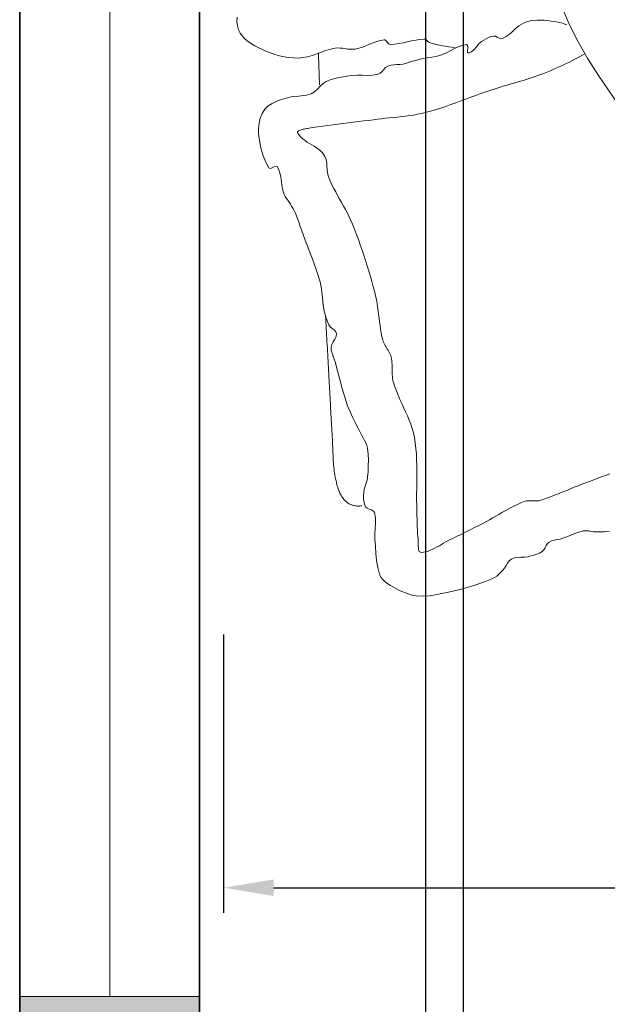
# Model space of a CAD drawing. Units: inches. Extents: x 2656 to 9931, y 1941 to 3068.
# Tile 6 of 46: x 2743 to 2773, y 2484 to 2533. Entities that reach past the tile are written whole.
import ezdxf

# ---------------------------------------------------------------- set-up
doc = ezdxf.new("R2010")
doc.units = ezdxf.units.IN
for name, color, linetype, lineweight in [('A-ANNO-DIMS', 2, 'Continuous', 18), ('A-FURN', 8, 'Continuous', 13), ('A-GLAZ', 4, 'Continuous', 18), ('A-WALL', 7, 'Continuous', 35), ('A-WALL-PATT', 251, 'Continuous', 13)]:
    doc.layers.add(name, color=color, linetype=linetype, lineweight=lineweight)
doc.styles.get("Standard").update_dxf_attribs({"font": 'arial.ttf'})
doc.dimstyles.new('ISO-25', dxfattribs={"dimtxt": 6, "dimasz": 2.5, "dimexe": 1.25, "dimexo": 0.625, "dimtad": 1, "dimdec": 0, "dimlunit": 3, "dimtxsty": 'Standard', "dimcen": 2.5, "dimadec": 0, "dimazin": 0, "dimtfac": 1, "dimtdec": 0, "dimtmove": 0, "dimatfit": 3, "dimfxl": 1, "dimarcsym": 0})

# ---------------------------------------------------------------- blocks, each defined once
blk = doc.blocks.new('BED-DOUBLE')
for p, q in [((16.849, 30.803), (17.238, 29.898)), ((0.636, 30.241), (0.624, 30.023)), ((15.288, 30.055), (15.465, 30.077)), ((15.465, 30.077), (15.645, 30.088)), ((15.645, 30.088), (15.823, 30.093)), ((15.823, 30.093), (15.993, 30.09)), ((15.993, 30.09), (16.162, 30.075)), ((16.162, 30.075), (16.331, 30.052)), ((0.624, 30.023), (0.642, 29.81)), ((0.642, 29.81), (0.701, 29.605)), ((0.701, 29.605), (0.788, 29.438)), ((14.332, 29.466), (14.528, 29.645)), ((14.528, 29.645), (14.729, 29.815)), ((14.729, 29.815), (14.951, 29.952)), ((14.951, 29.952), (15.115, 30.015)), ((15.115, 30.015), (15.288, 30.055)), ((16.331, 30.052), (16.5, 30.023)), ((16.5, 30.023), (16.667, 29.993)), ((16.667, 29.993), (16.759, 29.975)), ((16.759, 29.975), (16.85, 29.954)), ((16.85, 29.954), (16.94, 29.928)), ((16.94, 29.928), (17.029, 29.899)), ((17.029, 29.899), (17.117, 29.867)), ((17.238, 29.898), (17.685, 29.016)), ((0.788, 29.438), (0.899, 29.287)), ((0.899, 29.287), (1.032, 29.151)), ((1.032, 29.151), (1.182, 29.027)), ((7.611, 29.024), (7.794, 29.077)), ((7.794, 29.077), (7.98, 29.112)), ((7.98, 29.112), (8.025, 29.107)), ((8.025, 29.107), (8.065, 29.082)), ((8.065, 29.082), (8.102, 29.045)), ((9.352, 29.052), (9.563, 29.094)), ((9.563, 29.094), (9.775, 29.126)), ((9.775, 29.126), (9.989, 29.144)), ((9.989, 29.144), (10.03, 29.139)), ((10.03, 29.139), (10.068, 29.122)), ((10.068, 29.122), (10.104, 29.096)), ((10.104, 29.096), (10.138, 29.066)), ((12.86, 29.025), (12.971, 29.097)), ((12.971, 29.097), (13.085, 29.165)), ((13.085, 29.165), (13.204, 29.223)), ((13.204, 29.223), (13.327, 29.269)), ((13.327, 29.269), (13.455, 29.297)), ((13.455, 29.297), (13.547, 29.286)), ((13.547, 29.286), (13.639, 29.244)), ((13.639, 29.244), (13.729, 29.194)), ((13.729, 29.194), (13.818, 29.162)), ((13.818, 29.162), (13.905, 29.17)), ((13.905, 29.17), (14.129, 29.301)), ((14.129, 29.301), (14.332, 29.466)), ((1.182, 29.027), (1.343, 28.914)), ((1.343, 28.914), (1.513, 28.813)), ((1.513, 28.813), (1.686, 28.721)), ((1.686, 28.721), (1.859, 28.637)), ((1.859, 28.637), (2.075, 28.541)), ((5.07, 28.574), (5.3, 28.643)), ((5.3, 28.643), (5.533, 28.692)), ((5.533, 28.692), (5.657, 28.702)), ((5.657, 28.702), (5.782, 28.699)), ((5.782, 28.699), (5.907, 28.685)), ((5.907, 28.685), (6.032, 28.668)), ((6.032, 28.668), (6.158, 28.65)), ((6.158, 28.65), (6.283, 28.638)), ((6.283, 28.638), (6.407, 28.635)), ((6.407, 28.635), (6.531, 28.647)), ((6.531, 28.647), (6.716, 28.689)), ((6.716, 28.689), (6.897, 28.747)), ((6.897, 28.747), (7.076, 28.815)), ((7.076, 28.815), (7.254, 28.887)), ((7.254, 28.887), (7.432, 28.958)), ((7.432, 28.958), (7.611, 29.024)), ((8.102, 29.045), (8.137, 29.001)), ((8.137, 29.001), (8.172, 28.956)), ((8.172, 28.956), (8.208, 28.917)), ((8.208, 28.917), (8.249, 28.889)), ((8.249, 28.889), (8.295, 28.879)), ((8.295, 28.879), (8.508, 28.892)), ((8.508, 28.892), (8.72, 28.921)), ((8.72, 28.921), (8.931, 28.961)), ((8.931, 28.961), (9.142, 29.006)), ((9.142, 29.006), (9.352, 29.052)), ((10.138, 29.066), (10.173, 29.034)), ((10.173, 29.034), (10.208, 29.004)), ((10.208, 29.004), (10.245, 28.979)), ((10.245, 28.979), (10.285, 28.962)), ((10.285, 28.962), (10.438, 28.921)), ((10.438, 28.921), (10.592, 28.883)), ((10.592, 28.883), (10.747, 28.848)), ((10.747, 28.848), (10.902, 28.816)), ((10.902, 28.816), (11.058, 28.787)), ((11.058, 28.787), (11.214, 28.761)), ((11.214, 28.761), (11.371, 28.738)), ((11.318, 28.576), (11.574, 28.708)), ((11.371, 28.738), (11.528, 28.717)), ((11.574, 28.708), (11.835, 28.814)), ((11.835, 28.814), (12.108, 28.869)), ((12.108, 28.869), (12.16, 28.826)), ((12.164, 28.715), (12.151, 28.582)), ((12.151, 28.582), (12.154, 28.476)), ((12.16, 28.826), (12.164, 28.715)), ((12.36, 28.509), (12.49, 28.625)), ((12.49, 28.625), (12.608, 28.765)), ((12.608, 28.765), (12.727, 28.906)), ((12.727, 28.906), (12.86, 29.025)), ((17.685, 29.016), (18.177, 28.157)), ((2.075, 28.541), (2.296, 28.454)), ((2.296, 28.454), (2.522, 28.379)), ((2.522, 28.379), (2.752, 28.315)), ((2.752, 28.315), (2.985, 28.264)), ((2.985, 28.264), (3.219, 28.227)), ((3.219, 28.227), (3.455, 28.205)), ((3.455, 28.205), (3.69, 28.2)), ((3.69, 28.2), (3.926, 28.22)), ((3.926, 28.22), (4.158, 28.267)), ((4.158, 28.267), (4.387, 28.334)), ((4.387, 28.334), (4.615, 28.412)), ((4.615, 28.412), (4.842, 28.495)), ((4.7, 28.368), (4.698, 28.448)), ((4.703, 28.288), (4.7, 28.368)), ((4.706, 28.209), (4.703, 28.288)), ((4.709, 28.129), (4.706, 28.209)), ((4.712, 28.049), (4.709, 28.129)), ((4.842, 28.495), (5.07, 28.574)), ((9.564, 28.082), (9.721, 28.124)), ((9.721, 28.124), (9.937, 28.168)), ((9.937, 28.168), (10.154, 28.204)), ((10.154, 28.204), (10.371, 28.24)), ((10.371, 28.24), (10.586, 28.283)), ((10.586, 28.283), (10.798, 28.339)), ((10.798, 28.339), (11.062, 28.445)), ((11.062, 28.445), (11.318, 28.576)), ((12.154, 28.476), (12.205, 28.442)), ((12.205, 28.442), (12.36, 28.509)), ((17.373, 28.061), (17.53, 28.142)), ((17.53, 28.142), (17.686, 28.224)), ((17.686, 28.224), (17.841, 28.308)), ((17.841, 28.308), (17.995, 28.394)), ((18.177, 28.157), (18.699, 27.32)), ((4.715, 27.969), (4.712, 28.049)), ((4.717, 27.889), (4.715, 27.969)), ((4.72, 27.81), (4.717, 27.889)), ((4.723, 27.73), (4.72, 27.81)), ((4.726, 27.65), (4.723, 27.73)), ((4.728, 27.57), (4.726, 27.65)), ((7.882, 27.53), (7.969, 27.632)), ((7.969, 27.632), (8.06, 27.726)), ((8.06, 27.726), (8.166, 27.794)), ((8.166, 27.794), (8.314, 27.837)), ((8.314, 27.837), (8.468, 27.857)), ((8.468, 27.857), (8.625, 27.867)), ((8.625, 27.867), (8.782, 27.876)), ((8.782, 27.876), (8.937, 27.898)), ((8.937, 27.898), (9.095, 27.938)), ((9.095, 27.938), (9.252, 27.984)), ((9.252, 27.984), (9.408, 28.034)), ((9.408, 28.034), (9.564, 28.082)), ((16.25, 27.546), (16.413, 27.614)), ((16.413, 27.614), (16.575, 27.684)), ((16.575, 27.684), (16.736, 27.756)), ((16.736, 27.756), (16.897, 27.83)), ((16.897, 27.83), (17.056, 27.905)), ((17.056, 27.905), (17.215, 27.982)), ((17.215, 27.982), (17.373, 28.061)), ((4.731, 27.49), (4.728, 27.57)), ((4.734, 27.41), (4.731, 27.49)), ((4.737, 27.331), (4.734, 27.41)), ((4.74, 27.251), (4.737, 27.331)), ((4.743, 27.171), (4.74, 27.251)), ((4.745, 27.091), (4.743, 27.171)), ((5.093, 27.032), (5.338, 27.125)), ((5.338, 27.125), (5.592, 27.193)), ((5.592, 27.193), (5.851, 27.245)), ((5.851, 27.245), (6.113, 27.285)), ((6.113, 27.285), (6.374, 27.321)), ((6.374, 27.321), (6.635, 27.34)), ((6.635, 27.34), (6.898, 27.338)), ((6.898, 27.338), (7.162, 27.333)), ((7.162, 27.333), (7.422, 27.343)), ((7.422, 27.343), (7.678, 27.387)), ((7.678, 27.387), (7.789, 27.442)), ((7.789, 27.442), (7.882, 27.53)), ((14.933, 27.081), (15.133, 27.143)), ((15.133, 27.143), (15.332, 27.207)), ((15.332, 27.207), (15.53, 27.273)), ((15.53, 27.273), (15.727, 27.343)), ((15.727, 27.343), (15.923, 27.416)), ((15.923, 27.416), (16.087, 27.48)), ((16.087, 27.48), (16.25, 27.546)), ((18.699, 27.32), (19.702, 25.863)), ((4.501, 26.512), (4.646, 26.646)), ((4.646, 26.646), (4.784, 26.793)), ((4.748, 27.011), (4.745, 27.091)), ((4.751, 26.932), (4.748, 27.011)), ((4.754, 26.852), (4.751, 26.932)), ((4.784, 26.793), (4.929, 26.929)), ((4.929, 26.929), (5.093, 27.032)), ((13.332, 26.597), (13.531, 26.661)), ((13.531, 26.661), (13.73, 26.724)), ((13.73, 26.724), (13.93, 26.784)), ((13.93, 26.784), (14.131, 26.844)), ((14.131, 26.844), (14.332, 26.903)), ((14.332, 26.903), (14.532, 26.961)), ((14.532, 26.961), (14.733, 27.021)), ((14.733, 27.021), (14.933, 27.081)), ((2.617, 26.032), (2.853, 26.116)), ((2.853, 26.116), (3.086, 26.193)), ((3.086, 26.193), (3.333, 26.252)), ((3.333, 26.252), (3.587, 26.281)), ((3.587, 26.281), (3.842, 26.303)), ((3.842, 26.303), (4.094, 26.34)), ((4.094, 26.34), (4.335, 26.412)), ((4.335, 26.412), (4.501, 26.512)), ((11.822, 26.049), (12.073, 26.143)), ((12.073, 26.143), (12.324, 26.237)), ((12.324, 26.237), (12.575, 26.33)), ((12.575, 26.33), (12.826, 26.422)), ((12.826, 26.422), (13.078, 26.511)), ((13.078, 26.511), (13.332, 26.597)), ((1.884, 25.422), (2.018, 25.634)), ((2.018, 25.634), (2.187, 25.802)), ((2.187, 25.802), (2.391, 25.931)), ((2.391, 25.931), (2.617, 26.032)), ((10.558, 25.613), (10.813, 25.693)), ((10.813, 25.693), (11.067, 25.778)), ((11.067, 25.778), (11.319, 25.866)), ((11.319, 25.866), (11.571, 25.957)), ((11.571, 25.957), (11.822, 26.049)), ((1.729, 24.935), (1.788, 25.186)), ((1.788, 25.186), (1.884, 25.422)), ((7.459, 25.114), (7.658, 25.139)), ((7.658, 25.139), (7.858, 25.162)), ((7.858, 25.162), (8.058, 25.184)), ((8.058, 25.184), (8.258, 25.204)), ((8.258, 25.204), (8.458, 25.224)), ((8.458, 25.224), (8.658, 25.245)), ((8.658, 25.245), (8.858, 25.267)), ((8.858, 25.267), (9.058, 25.291)), ((9.058, 25.291), (9.257, 25.318)), ((9.257, 25.318), (9.455, 25.348)), ((9.455, 25.348), (9.652, 25.383)), ((9.652, 25.383), (9.849, 25.423)), ((9.849, 25.423), (10.044, 25.469)), ((10.044, 25.469), (10.302, 25.538)), ((10.302, 25.538), (10.558, 25.613)), ((1.701, 24.678), (1.729, 24.935)), ((1.704, 24.424), (1.701, 24.678)), ((3.945, 24.636), (4.002, 24.647)), ((4.002, 24.647), (4.058, 24.657)), ((4.058, 24.657), (4.109, 24.665)), ((4.109, 24.665), (4.154, 24.673)), ((4.154, 24.673), (4.407, 24.716)), ((4.407, 24.716), (4.66, 24.756)), ((4.66, 24.756), (4.914, 24.794)), ((4.914, 24.794), (5.168, 24.829)), ((5.168, 24.829), (5.422, 24.863)), ((5.422, 24.863), (5.676, 24.895)), ((5.676, 24.895), (5.931, 24.926)), ((5.931, 24.926), (6.186, 24.957)), ((6.186, 24.957), (6.44, 24.987)), ((6.44, 24.987), (6.695, 25.017)), ((6.695, 25.017), (6.95, 25.048)), ((6.95, 25.048), (7.204, 25.081)), ((7.204, 25.081), (7.459, 25.114)), ((1.743, 24.066), (1.704, 24.424)), ((3.648, 24.471), (3.65, 24.502)), ((3.662, 24.438), (3.648, 24.471)), ((3.65, 24.502), (3.667, 24.529)), ((3.737, 24.332), (3.662, 24.438)), ((3.667, 24.529), (3.695, 24.553)), ((3.695, 24.553), (3.733, 24.574)), ((3.733, 24.574), (3.779, 24.593)), ((3.825, 24.237), (3.737, 24.332)), ((3.779, 24.593), (3.831, 24.609)), ((3.922, 24.151), (3.825, 24.237)), ((3.831, 24.609), (3.887, 24.623)), ((3.887, 24.623), (3.945, 24.636)), ((4.027, 24.071), (3.922, 24.151)), ((1.814, 23.71), (1.743, 24.066)), ((1.915, 23.361), (1.814, 23.71)), ((4.138, 23.996), (4.027, 24.071)), ((4.252, 23.924), (4.138, 23.996)), ((4.367, 23.854), (4.252, 23.924)), ((4.482, 23.783), (4.367, 23.854)), ((4.594, 23.709), (4.482, 23.783)), ((4.702, 23.631), (4.594, 23.709)), ((2.047, 23.023), (1.915, 23.361)), ((4.803, 23.547), (4.702, 23.631)), ((4.895, 23.455), (4.803, 23.547)), ((4.976, 23.353), (4.895, 23.455)), ((5.021, 23.278), (4.976, 23.353)), ((5.055, 23.198), (5.021, 23.278)), ((5.08, 23.115), (5.055, 23.198)), ((2.209, 22.702), (2.047, 23.023)), ((2.277, 22.669), (2.209, 22.702)), ((2.376, 22.698), (2.277, 22.669)), ((2.486, 22.749), (2.376, 22.698)), ((2.586, 22.779), (2.486, 22.749)), ((2.655, 22.747), (2.586, 22.779)), ((2.758, 22.509), (2.655, 22.747)), ((5.098, 23.029), (5.08, 23.115)), ((5.11, 22.94), (5.098, 23.029)), ((5.118, 22.85), (5.11, 22.94)), ((5.124, 22.758), (5.118, 22.85)), ((5.129, 22.666), (5.124, 22.758)), ((5.136, 22.575), (5.129, 22.666)), ((2.814, 22.253), (2.758, 22.509)), ((2.848, 21.988), (2.814, 22.253)), ((5.146, 22.484), (5.136, 22.575)), ((5.16, 22.395), (5.146, 22.484)), ((5.181, 22.309), (5.16, 22.395)), ((5.21, 22.225), (5.181, 22.309)), ((5.29, 22.04), (5.21, 22.225)), ((2.883, 21.722), (2.848, 21.988)), ((2.944, 21.465), (2.883, 21.722)), ((5.376, 21.857), (5.29, 22.04)), ((5.467, 21.676), (5.376, 21.857)), ((2.987, 21.364), (2.944, 21.465)), ((3.042, 21.269), (2.987, 21.364)), ((3.105, 21.176), (3.042, 21.269)), ((5.562, 21.498), (5.467, 21.676)), ((5.659, 21.32), (5.562, 21.498)), ((5.758, 21.144), (5.659, 21.32)), ((3.17, 21.085), (3.105, 21.176)), ((3.23, 20.991), (3.17, 21.085)), ((3.294, 20.888), (3.23, 20.991)), ((3.358, 20.785), (3.294, 20.888)), ((3.422, 20.681), (3.358, 20.785)), ((5.858, 20.967), (5.758, 21.144)), ((5.956, 20.79), (5.858, 20.967)), ((6.053, 20.612), (5.956, 20.79)), ((3.482, 20.575), (3.422, 20.681)), ((3.535, 20.466), (3.482, 20.575)), ((3.605, 20.296), (3.535, 20.466)), ((3.669, 20.123), (3.605, 20.296)), ((6.147, 20.433), (6.053, 20.612)), ((6.237, 20.253), (6.147, 20.433)), ((6.322, 20.069), (6.237, 20.253)), ((3.729, 19.948), (3.669, 20.123)), ((3.787, 19.772), (3.729, 19.948)), ((3.848, 19.598), (3.787, 19.772)), ((6.401, 19.883), (6.322, 20.069)), ((6.502, 19.627), (6.401, 19.883)), ((4.042, 19.079), (3.848, 19.598)), ((6.6, 19.369), (6.502, 19.627)), ((6.696, 19.11), (6.6, 19.369)), ((4.241, 18.561), (4.042, 19.079)), ((6.789, 18.85), (6.696, 19.11)), ((6.88, 18.59), (6.789, 18.85)), ((4.437, 18.043), (4.241, 18.561)), ((6.968, 18.328), (6.88, 18.59)), ((7.053, 18.065), (6.968, 18.328)), ((4.623, 17.521), (4.437, 18.043)), ((7.136, 17.802), (7.053, 18.065)), ((7.217, 17.538), (7.136, 17.802)), ((4.788, 16.993), (4.623, 17.521)), ((7.295, 17.273), (7.217, 17.538)), ((7.37, 17.008), (7.295, 17.273)), ((4.842, 16.744), (4.788, 16.993)), ((7.443, 16.742), (7.37, 17.008)), ((4.873, 16.49), (4.842, 16.744)), ((4.894, 16.234), (4.873, 16.49)), ((7.514, 16.475), (7.443, 16.742)), ((7.558, 16.293), (7.514, 16.475)), ((7.596, 16.111), (7.558, 16.293)), ((4.918, 15.978), (4.894, 16.234)), ((4.956, 15.726), (4.918, 15.978)), ((7.628, 15.927), (7.596, 16.111)), ((7.656, 15.742), (7.628, 15.927)), ((4.993, 15.544), (4.956, 15.726)), ((5.035, 15.362), (4.993, 15.544)), ((5.084, 15.183), (5.035, 15.362)), ((5.061, 15.137), (5.052, 15.298)), ((7.682, 15.557), (7.656, 15.742)), ((7.706, 15.371), (7.682, 15.557)), ((7.729, 15.185), (7.706, 15.371)), ((5.071, 14.976), (5.061, 15.137)), ((5.08, 14.815), (5.071, 14.976)), ((5.089, 14.653), (5.08, 14.815)), ((5.144, 15.008), (5.084, 15.183)), ((5.218, 14.839), (5.144, 15.008)), ((5.29, 14.745), (5.218, 14.839)), ((7.753, 14.999), (7.729, 15.185)), ((7.778, 14.814), (7.753, 14.999)), ((7.806, 14.629), (7.778, 14.814)), ((5.098, 14.492), (5.089, 14.653)), ((5.107, 14.331), (5.098, 14.492)), ((5.116, 14.17), (5.107, 14.331)), ((5.386, 14.665), (5.29, 14.745)), ((5.486, 14.589), (5.386, 14.665)), ((5.567, 14.505), (5.486, 14.589)), ((5.607, 14.402), (5.567, 14.505)), ((5.588, 14.261), (5.607, 14.402)), ((7.837, 14.445), (7.806, 14.629)), ((7.874, 14.262), (7.837, 14.445)), ((5.125, 14.008), (5.116, 14.17)), ((5.135, 13.847), (5.125, 14.008)), ((5.144, 13.686), (5.135, 13.847)), ((5.331, 13.725), (5.367, 13.865)), ((5.367, 13.865), (5.44, 13.998)), ((5.44, 13.998), (5.524, 14.129)), ((5.524, 14.129), (5.588, 14.261)), ((7.916, 14.08), (7.874, 14.262)), ((7.937, 14.012), (7.916, 14.08)), ((7.963, 13.946), (7.937, 14.012)), ((7.994, 13.881), (7.963, 13.946)), ((8.029, 13.818), (7.994, 13.881)), ((8.066, 13.756), (8.029, 13.818)), ((5.153, 13.525), (5.144, 13.686)), ((5.162, 13.363), (5.153, 13.525)), ((5.171, 13.202), (5.162, 13.363)), ((5.341, 13.575), (5.331, 13.725)), ((5.379, 13.427), (5.341, 13.575)), ((5.432, 13.282), (5.379, 13.427)), ((8.105, 13.695), (8.066, 13.756)), ((8.144, 13.633), (8.105, 13.695)), ((8.182, 13.572), (8.144, 13.633)), ((8.219, 13.51), (8.182, 13.572)), ((8.254, 13.447), (8.219, 13.51)), ((8.285, 13.382), (8.254, 13.447)), ((8.311, 13.316), (8.285, 13.382)), ((8.332, 13.248), (8.311, 13.316)), ((5.18, 13.041), (5.171, 13.202)), ((5.189, 12.88), (5.18, 13.041)), ((5.198, 12.718), (5.189, 12.88)), ((5.489, 13.137), (5.432, 13.282)), ((5.538, 12.991), (5.489, 13.137)), ((5.657, 12.549), (5.538, 12.991)), ((8.352, 13.151), (8.332, 13.248)), ((8.367, 13.053), (8.352, 13.151)), ((8.376, 12.954), (8.367, 13.053)), ((8.381, 12.855), (8.376, 12.954)), ((8.383, 12.755), (8.381, 12.855)), ((5.207, 12.557), (5.198, 12.718)), ((5.216, 12.396), (5.207, 12.557)), ((5.225, 12.235), (5.216, 12.396)), ((5.771, 12.106), (5.657, 12.549)), ((8.384, 12.654), (8.383, 12.755)), ((8.385, 12.554), (8.384, 12.654)), ((8.387, 12.454), (8.385, 12.554)), ((8.39, 12.354), (8.387, 12.454)), ((8.397, 12.255), (8.39, 12.354)), ((5.234, 12.073), (5.225, 12.235)), ((5.242, 11.932), (5.234, 12.073)), ((5.249, 11.79), (5.242, 11.932)), ((5.888, 11.664), (5.771, 12.106)), ((8.408, 12.156), (8.397, 12.255)), ((8.425, 12.059), (8.408, 12.156)), ((8.449, 11.963), (8.425, 12.059)), ((8.517, 11.748), (8.449, 11.963)), ((5.257, 11.649), (5.249, 11.79)), ((5.264, 11.507), (5.257, 11.649)), ((5.272, 11.366), (5.264, 11.507)), ((5.279, 11.224), (5.272, 11.366)), ((6.014, 11.224), (5.888, 11.664)), ((8.595, 11.536), (8.517, 11.748)), ((8.68, 11.326), (8.595, 11.536)), ((5.286, 11.083), (5.279, 11.224)), ((5.294, 10.941), (5.286, 11.083)), ((5.301, 10.8), (5.294, 10.941)), ((6.158, 10.79), (6.014, 11.224)), ((8.771, 11.118), (8.68, 11.326)), ((8.865, 10.911), (8.771, 11.118)), ((8.96, 10.704), (8.865, 10.911)), ((5.309, 10.658), (5.301, 10.8)), ((5.316, 10.516), (5.309, 10.658)), ((5.323, 10.375), (5.316, 10.516)), ((5.331, 10.233), (5.323, 10.375)), ((6.281, 10.487), (6.158, 10.79)), ((6.42, 10.191), (6.281, 10.487)), ((9.055, 10.498), (8.96, 10.704)), ((9.147, 10.291), (9.055, 10.498)), ((5.339, 10.092), (5.331, 10.233)), ((5.347, 9.95), (5.339, 10.092)), ((5.355, 9.809), (5.347, 9.95)), ((6.569, 9.899), (6.42, 10.191)), ((6.72, 9.607), (6.569, 9.899)), ((9.235, 10.082), (9.147, 10.291)), ((9.315, 9.872), (9.235, 10.082)), ((9.387, 9.659), (9.315, 9.872)), ((5.363, 9.667), (5.355, 9.809)), ((5.371, 9.526), (5.363, 9.667)), ((5.38, 9.384), (5.371, 9.526)), ((5.389, 9.243), (5.38, 9.384)), ((6.864, 9.313), (6.72, 9.607)), ((9.447, 9.442), (9.387, 9.659)), ((9.495, 9.223), (9.447, 9.442)), ((5.395, 9.142), (5.389, 9.243)), ((5.4, 9.04), (5.395, 9.142)), ((5.404, 8.939), (5.4, 9.04)), ((5.408, 8.837), (5.404, 8.939)), ((6.93, 9.186), (6.864, 9.313)), ((7, 9.061), (6.93, 9.186)), ((7.067, 8.934), (7, 9.061)), ((7.122, 8.804), (7.067, 8.934)), ((9.539, 8.941), (9.495, 9.223)), ((9.573, 8.659), (9.539, 8.941)), ((5.412, 8.735), (5.408, 8.837)), ((5.416, 8.634), (5.412, 8.735)), ((5.419, 8.532), (5.416, 8.634)), ((5.423, 8.43), (5.419, 8.532)), ((5.427, 8.329), (5.423, 8.43)), ((7.155, 8.667), (7.122, 8.804)), ((7.184, 8.38), (7.155, 8.667)), ((7.195, 8.092), (7.184, 8.38)), ((9.596, 8.375), (9.573, 8.659)), ((5.432, 8.227), (5.427, 8.329)), ((5.437, 8.125), (5.432, 8.227)), ((5.443, 8.024), (5.437, 8.125)), ((5.45, 7.923), (5.443, 8.024)), ((5.458, 7.822), (5.45, 7.923)), ((7.192, 7.802), (7.195, 8.092)), ((9.611, 8.09), (9.596, 8.375)), ((9.62, 7.805), (9.611, 8.09)), ((5.468, 7.721), (5.458, 7.822)), ((5.479, 7.62), (5.468, 7.721)), ((5.492, 7.52), (5.479, 7.62)), ((5.506, 7.419), (5.492, 7.52)), ((5.522, 7.319), (5.506, 7.419)), ((7.156, 7.225), (7.178, 7.513)), ((7.178, 7.513), (7.192, 7.802)), ((9.622, 7.519), (9.62, 7.805)), ((9.621, 7.233), (9.622, 7.519)), ((5.541, 7.22), (5.522, 7.319)), ((5.553, 7.158), (5.541, 7.22)), ((5.566, 7.096), (5.553, 7.158)), ((5.58, 7.034), (5.566, 7.096)), ((5.594, 6.972), (5.58, 7.034)), ((5.609, 6.909), (5.594, 6.972)), ((5.626, 6.847), (5.609, 6.909)), ((7.035, 6.769), (7.085, 6.92)), ((7.085, 6.92), (7.129, 7.071)), ((7.129, 7.071), (7.156, 7.225)), ((9.614, 6.66), (9.618, 6.946)), ((9.618, 6.946), (9.621, 7.233)), ((18.066, 6.943), (17.874, 6.869)), ((18.258, 7.014), (18.066, 6.943)), ((18.383, 7.06), (18.258, 7.014)), ((18.509, 7.107), (18.383, 7.06)), ((18.634, 7.155), (18.509, 7.107)), ((18.76, 7.204), (18.634, 7.155)), ((18.885, 7.251), (18.76, 7.204)), ((19.011, 7.298), (18.885, 7.251)), ((19.137, 7.343), (19.011, 7.298)), ((19.264, 7.386), (19.137, 7.343)), ((5.643, 6.785), (5.626, 6.847)), ((5.661, 6.724), (5.643, 6.785)), ((5.681, 6.663), (5.661, 6.724)), ((5.702, 6.603), (5.681, 6.663)), ((5.725, 6.543), (5.702, 6.603)), ((5.749, 6.484), (5.725, 6.543)), ((5.776, 6.427), (5.749, 6.484)), ((5.804, 6.37), (5.776, 6.427)), ((6.96, 6.317), (6.968, 6.464)), ((6.968, 6.464), (6.992, 6.618)), ((6.992, 6.618), (7.035, 6.769)), ((9.611, 6.373), (9.614, 6.66)), ((16.735, 6.407), (16.545, 6.332)), ((16.925, 6.483), (16.735, 6.407)), ((17.115, 6.561), (16.925, 6.483)), ((17.304, 6.639), (17.115, 6.561)), ((17.494, 6.717), (17.304, 6.639)), ((17.684, 6.794), (17.494, 6.717)), ((17.874, 6.869), (17.684, 6.794)), ((5.833, 6.315), (5.804, 6.37)), ((5.865, 6.261), (5.833, 6.315)), ((5.899, 6.209), (5.865, 6.261)), ((5.936, 6.159), (5.899, 6.209)), ((5.975, 6.11), (5.936, 6.159)), ((6.016, 6.063), (5.975, 6.11)), ((6.047, 6.031), (6.016, 6.063)), ((6.081, 6.001), (6.047, 6.031)), ((6.116, 5.972), (6.081, 6.001)), ((6.154, 5.945), (6.116, 5.972)), ((6.193, 5.92), (6.154, 5.945)), ((6.233, 5.897), (6.193, 5.92)), ((6.959, 6.168), (6.96, 6.317)), ((6.97, 6.021), (6.959, 6.168)), ((7, 5.878), (6.97, 6.021)), ((9.609, 6.087), (9.611, 6.373)), ((9.612, 5.801), (9.609, 6.087)), ((14.821, 5.938), (14.66, 5.864)), ((14.984, 6.007), (14.821, 5.938)), ((15.041, 6.026), (14.984, 6.007)), ((15.1, 6.038), (15.041, 6.026)), ((15.16, 6.045), (15.1, 6.038)), ((15.221, 6.047), (15.16, 6.045)), ((15.282, 6.046), (15.221, 6.047)), ((15.344, 6.043), (15.282, 6.046)), ((15.407, 6.039), (15.344, 6.043)), ((15.469, 6.035), (15.407, 6.039)), ((15.531, 6.033), (15.469, 6.035)), ((15.593, 6.033), (15.531, 6.033)), ((15.654, 6.037), (15.593, 6.033)), ((15.714, 6.046), (15.654, 6.037)), ((15.773, 6.06), (15.714, 6.046)), ((15.968, 6.123), (15.773, 6.06)), ((16.161, 6.189), (15.968, 6.123)), ((16.354, 6.259), (16.161, 6.189)), ((16.545, 6.332), (16.354, 6.259)), ((6.275, 5.876), (6.233, 5.897)), ((6.318, 5.856), (6.275, 5.876)), ((6.362, 5.839), (6.318, 5.856)), ((6.407, 5.823), (6.362, 5.839)), ((6.452, 5.81), (6.407, 5.823)), ((6.498, 5.798), (6.452, 5.81)), ((6.544, 5.789), (6.498, 5.798)), ((6.591, 5.783), (6.544, 5.789)), ((6.637, 5.778), (6.591, 5.783)), ((6.684, 5.776), (6.637, 5.778)), ((6.73, 5.776), (6.684, 5.776)), ((6.775, 5.779), (6.73, 5.776)), ((6.82, 5.784), (6.775, 5.779)), ((6.864, 5.792), (6.82, 5.784)), ((7.054, 5.745), (7, 5.878)), ((7.129, 5.669), (7.054, 5.745)), ((7.236, 5.621), (7.129, 5.669)), ((7.351, 5.581), (7.236, 5.621)), ((7.45, 5.529), (7.351, 5.581)), ((7.508, 5.447), (7.45, 5.529)), ((7.553, 5.189), (7.508, 5.447)), ((9.619, 5.515), (9.612, 5.801)), ((9.623, 5.402), (9.619, 5.515)), ((13.878, 5.447), (13.724, 5.359)), ((14.032, 5.535), (13.878, 5.447)), ((14.187, 5.621), (14.032, 5.535)), ((14.343, 5.705), (14.187, 5.621)), ((14.501, 5.787), (14.343, 5.705)), ((14.66, 5.864), (14.501, 5.787)), ((7.556, 4.925), (7.553, 5.189)), ((9.627, 5.288), (9.623, 5.402)), ((9.63, 5.174), (9.627, 5.288)), ((9.633, 5.061), (9.63, 5.174)), ((9.636, 4.947), (9.633, 5.061)), ((9.64, 4.833), (9.636, 4.947)), ((13.106, 5.009), (12.949, 4.926)), ((13.261, 5.095), (13.106, 5.009)), ((13.416, 5.182), (13.261, 5.095)), ((13.57, 5.27), (13.416, 5.182)), ((13.724, 5.359), (13.57, 5.27)), ((7.52, 4.39), (7.538, 4.658)), ((7.538, 4.658), (7.556, 4.925)), ((9.644, 4.72), (9.64, 4.833)), ((9.648, 4.606), (9.644, 4.72)), ((9.654, 4.493), (9.648, 4.606)), ((9.661, 4.379), (9.654, 4.493)), ((12.057, 4.472), (11.929, 4.408)), ((12.185, 4.536), (12.057, 4.472)), ((12.313, 4.6), (12.185, 4.536)), ((12.44, 4.665), (12.313, 4.6)), ((12.567, 4.73), (12.44, 4.665)), ((12.695, 4.795), (12.567, 4.73)), ((12.822, 4.861), (12.695, 4.795)), ((12.949, 4.926), (12.822, 4.861)), ((17.73, 4.479), (17.526, 4.406)), ((17.94, 4.533), (17.73, 4.479)), ((18.07, 4.542), (17.94, 4.533)), ((18.2, 4.53), (18.07, 4.542)), ((18.331, 4.508), (18.2, 4.53)), ((18.463, 4.487), (18.331, 4.508)), ((18.594, 4.48), (18.463, 4.487)), ((18.808, 4.485), (18.594, 4.48)), ((19.022, 4.492), (18.808, 4.485)), ((19.236, 4.507), (19.022, 4.492)), ((7.523, 4.124), (7.52, 4.39)), ((7.547, 3.768), (7.523, 4.124)), ((9.669, 4.266), (9.661, 4.379)), ((9.678, 4.153), (9.669, 4.266)), ((9.69, 4.04), (9.678, 4.153)), ((9.693, 3.991), (9.69, 4.04)), ((9.694, 3.937), (9.693, 3.991)), ((11.068, 3.982), (10.96, 3.92)), ((11.176, 4.041), (11.068, 3.982)), ((11.286, 4.096), (11.176, 4.041)), ((11.415, 4.157), (11.286, 4.096)), ((11.544, 4.219), (11.415, 4.157)), ((11.672, 4.281), (11.544, 4.219)), ((11.801, 4.344), (11.672, 4.281)), ((11.929, 4.408), (11.801, 4.344)), ((16.236, 3.976), (16.152, 3.897)), ((16.362, 4.037), (16.236, 3.976)), ((16.497, 4.076), (16.362, 4.037)), ((16.638, 4.103), (16.497, 4.076)), ((16.78, 4.129), (16.638, 4.103)), ((16.918, 4.164), (16.78, 4.129)), ((17.123, 4.239), (16.918, 4.164)), ((17.324, 4.323), (17.123, 4.239)), ((17.526, 4.406), (17.324, 4.323)), ((7.571, 3.41), (7.547, 3.768)), ((9.694, 3.879), (9.694, 3.937)), ((9.694, 3.819), (9.694, 3.879)), ((9.694, 3.759), (9.694, 3.819)), ((9.696, 3.701), (9.694, 3.759)), ((9.701, 3.645), (9.696, 3.701)), ((9.71, 3.593), (9.701, 3.645)), ((9.723, 3.548), (9.71, 3.593)), ((9.741, 3.51), (9.723, 3.548)), ((9.767, 3.482), (9.741, 3.51)), ((9.8, 3.464), (9.767, 3.482)), ((9.841, 3.459), (9.8, 3.464)), ((9.961, 3.47), (9.841, 3.459)), ((10.078, 3.492), (9.961, 3.47)), ((10.193, 3.525), (10.078, 3.492)), ((10.306, 3.567), (10.193, 3.525)), ((10.418, 3.616), (10.306, 3.567)), ((10.528, 3.671), (10.418, 3.616)), ((10.636, 3.73), (10.528, 3.671)), ((10.745, 3.793), (10.636, 3.73)), ((10.852, 3.856), (10.745, 3.793)), ((10.96, 3.92), (10.852, 3.856)), ((15.887, 3.503), (15.756, 3.427)), ((15.969, 3.585), (15.887, 3.503)), ((16.032, 3.687), (15.969, 3.585)), ((16.088, 3.796), (16.032, 3.687)), ((16.152, 3.897), (16.088, 3.796)), ((7.605, 3.054), (7.571, 3.41)), ((7.663, 2.703), (7.605, 3.054)), ((14.241, 3.037), (14.156, 2.925)), ((14.35, 3.122), (14.241, 3.037)), ((14.503, 3.18), (14.35, 3.122)), ((14.667, 3.204), (14.503, 3.18)), ((14.836, 3.212), (14.667, 3.204)), ((15.006, 3.22), (14.836, 3.212)), ((15.171, 3.245), (15.006, 3.22)), ((15.32, 3.282), (15.171, 3.245)), ((15.469, 3.321), (15.32, 3.282)), ((15.615, 3.368), (15.469, 3.321)), ((15.756, 3.427), (15.615, 3.368)), ((7.755, 2.361), (7.663, 2.703)), ((13.917, 2.562), (13.819, 2.464)), ((14.006, 2.674), (13.917, 2.562)), ((14.081, 2.799), (14.006, 2.674)), ((14.156, 2.925), (14.081, 2.799)), ((7.822, 2.221), (7.755, 2.361)), ((7.918, 2.097), (7.822, 2.221)), ((8.036, 1.988), (7.918, 2.097)), ((8.166, 1.891), (8.036, 1.988)), ((12.951, 1.974), (12.518, 1.825)), ((13.378, 2.137), (12.951, 1.974)), ((13.5, 2.198), (13.378, 2.137)), ((13.613, 2.277), (13.5, 2.198)), ((13.719, 2.367), (13.613, 2.277)), ((13.819, 2.464), (13.719, 2.367)), ((8.301, 1.807), (8.166, 1.891)), ((8.543, 1.669), (8.301, 1.807)), ((8.793, 1.539), (8.543, 1.669)), ((9.05, 1.427), (8.793, 1.539)), ((11.64, 1.572), (11.195, 1.465)), ((12.081, 1.691), (11.64, 1.572)), ((12.518, 1.825), (12.081, 1.691)), ((9.313, 1.341), (9.05, 1.427)), ((9.585, 1.289), (9.313, 1.341)), ((9.908, 1.271), (9.585, 1.289)), ((10.231, 1.29), (9.908, 1.271)), ((10.555, 1.334), (10.231, 1.29)), ((10.877, 1.396), (10.555, 1.334)), ((11.195, 1.465), (10.877, 1.396))]:
    blk.add_line(p, q)
blk = doc.blocks.new('WIN-60IN-SASH')
blk.add_line((4.457, 0.033), (4.457, 60.033))
blk = doc.blocks.new('*D31')
at = {"layer": 'A-ANNO-DIMS', "color": 0, "lineweight": -2, "transparency": 16777216}
for p, q in [((2753.358, 2502.145), (2753.358, 2488.227)), ((2841.982, 2502.145), (2841.982, 2488.227)), ((2755.858, 2489.477), (2839.482, 2489.477)), ((2841.982, 2489.477), (2952.348, 2489.477))]:
    blk.add_line(p, q, dxfattribs=at)
at = {"layer": 'A-ANNO-DIMS', "color": 0, "transparency": 16777216}
for points in [[(2755.858, 2489.893), (2755.858, 2489.06), (2753.358, 2489.477)], [(2839.482, 2489.893), (2839.482, 2489.06), (2841.982, 2489.477)]]:
    blk.add_solid(points, dxfattribs=at)
at = {"layer": 'Defpoints', "color": 0, "transparency": 16777216}
for p in [(2753.358, 2502.77), (2841.982, 2502.77), (2841.982, 2489.477)]:
    blk.add_point(p, dxfattribs=at)
at = {"layer": 'A-ANNO-DIMS', "color": 0, "transparency": 16777216, "insert": (2898.415, 2493.206), "char_height": 6, "attachment_point": 5}
blk.add_mtext('DOUBLE BED 7\'-4 1/2" TYP.', dxfattribs=at)
blk = doc.blocks.new('*D113')
at = {"layer": 'A-ANNO-DIMS', "color": 0, "lineweight": -2, "transparency": 16777216}
for p, q in [((2752.157, 2300.725), (2752.157, 2674.45)), ((2809.769, 2300.725), (2809.769, 2674.45)), ((2754.657, 2673.2), (2807.269, 2673.2))]:
    blk.add_line(p, q, dxfattribs=at)
at = {"layer": 'A-ANNO-DIMS', "color": 0, "transparency": 16777216}
for points in [[(2754.657, 2673.617), (2754.657, 2672.784), (2752.157, 2673.2)], [(2807.269, 2673.617), (2807.269, 2672.784), (2809.769, 2673.2)]]:
    blk.add_solid(points, dxfattribs=at)
at = {"layer": 'Defpoints', "color": 0, "transparency": 16777216}
for p in [(2809.769, 2673.2), (2752.157, 2300.1), (2809.769, 2300.1)]:
    blk.add_point(p, dxfattribs=at)
at = {"layer": 'A-ANNO-DIMS', "color": 0, "transparency": 16777216, "insert": (2780.963, 2676.928), "char_height": 6, "attachment_point": 5}
blk.add_mtext('4\'-9 1/2"', dxfattribs=at)
blk = doc.blocks.new('*D129')
at = {"layer": 'A-ANNO-DIMS', "color": 0, "lineweight": -2, "transparency": 16777216}
for p, q in [((2752.157, 2601.146), (2752.157, 2009.273)), ((2777.587, 2557.74), (2777.587, 2009.273)), ((2754.657, 2010.523), (2775.087, 2010.523)), ((2777.587, 2010.523), (2811.37, 2010.523))]:
    blk.add_line(p, q, dxfattribs=at)
at = {"layer": 'A-ANNO-DIMS', "color": 0, "transparency": 16777216}
for points in [[(2754.657, 2010.939), (2754.657, 2010.106), (2752.157, 2010.523)], [(2775.087, 2010.939), (2775.087, 2010.106), (2777.587, 2010.523)]]:
    blk.add_solid(points, dxfattribs=at)
at = {"layer": 'Defpoints', "color": 0, "transparency": 16777216}
for p in [(2752.157, 2601.771), (2777.587, 2558.365), (2777.587, 2010.523)]:
    blk.add_point(p, dxfattribs=at)
at = {"layer": 'A-ANNO-DIMS', "color": 0, "transparency": 16777216, "insert": (2795.728, 2014.25), "char_height": 6, "attachment_point": 5}
blk.add_mtext('2\'-1 1/2"', dxfattribs=at)
blk = doc.blocks.new('*D132')
at = {"layer": 'A-ANNO-DIMS', "color": 0, "lineweight": -2, "transparency": 16777216}
for p, q in [((2763.467, 2366.557), (2763.467, 2674.45)), ((2805.965, 2366.557), (2805.965, 2674.45)), ((2765.967, 2673.2), (2803.465, 2673.2))]:
    blk.add_line(p, q, dxfattribs=at)
at = {"layer": 'A-ANNO-DIMS', "color": 0, "transparency": 16777216}
for points in [[(2765.967, 2673.617), (2765.967, 2672.784), (2763.467, 2673.2)], [(2803.465, 2673.617), (2803.465, 2672.784), (2805.965, 2673.2)]]:
    blk.add_solid(points, dxfattribs=at)
at = {"layer": 'Defpoints', "color": 0, "transparency": 16777216}
for p in [(2805.965, 2673.2), (2763.467, 2365.932), (2805.965, 2365.932)]:
    blk.add_point(p, dxfattribs=at)
at = {"layer": 'A-ANNO-DIMS', "color": 0, "transparency": 16777216, "insert": (2784.716, 2676.93), "char_height": 6, "attachment_point": 5}
blk.add_mtext('3\'-6 1/2"', dxfattribs=at)
blk = doc.blocks.new('*D134')
at = {"layer": 'A-ANNO-DIMS', "color": 0, "lineweight": -2, "transparency": 16777216}
for p, q in [((2752.157, 2300.725), (2752.157, 2674.45)), ((2763.467, 2347.433), (2763.467, 2674.45)), ((2754.657, 2673.2), (2760.967, 2673.2)), ((2763.467, 2673.2), (2801.809, 2673.2))]:
    blk.add_line(p, q, dxfattribs=at)
at = {"layer": 'A-ANNO-DIMS', "color": 0, "transparency": 16777216}
for points in [[(2754.657, 2673.617), (2754.657, 2672.784), (2752.157, 2673.2)], [(2760.967, 2673.617), (2760.967, 2672.784), (2763.467, 2673.2)]]:
    blk.add_solid(points, dxfattribs=at)
at = {"layer": 'Defpoints', "color": 0, "transparency": 16777216}
for p in [(2763.467, 2673.2), (2763.467, 2346.808), (2752.157, 2300.1)]:
    blk.add_point(p, dxfattribs=at)
at = {"layer": 'A-ANNO-DIMS', "color": 0, "transparency": 16777216, "insert": (2783.888, 2676.928), "char_height": 6, "attachment_point": 5}
blk.add_mtext('0\'-11 1/2"', dxfattribs=at)
blk = doc.blocks.new('*D136')
at = {"layer": 'A-ANNO-DIMS', "color": 0, "lineweight": -2, "transparency": 16777216}
for p, q in [((2765.357, 2375.042), (2765.357, 2674.45)), ((2779.142, 2375.042), (2779.142, 2674.45)), ((2767.857, 2673.2), (2776.642, 2673.2)), ((2779.142, 2673.2), (2798.277, 2673.2))]:
    blk.add_line(p, q, dxfattribs=at)
at = {"layer": 'A-ANNO-DIMS', "color": 0, "transparency": 16777216}
for points in [[(2767.857, 2673.617), (2767.857, 2672.784), (2765.357, 2673.2)], [(2776.642, 2673.617), (2776.642, 2672.784), (2779.142, 2673.2)]]:
    blk.add_solid(points, dxfattribs=at)
at = {"layer": 'Defpoints', "color": 0, "transparency": 16777216}
for p in [(2779.142, 2673.2), (2765.357, 2374.417), (2779.142, 2374.417)]:
    blk.add_point(p, dxfattribs=at)
at = {"layer": 'A-ANNO-DIMS', "color": 0, "transparency": 16777216, "insert": (2789.959, 2676.838), "char_height": 6, "attachment_point": 5}
blk.add_mtext('1\'-2"', dxfattribs=at)

msp = doc.modelspace()

# ---------------------------------------------------------------- hatches: boundary and pattern name
at = {"layer": 'A-WALL-PATT'}
h = msp.add_hatch(color=256, dxfattribs=at)
h.dxf.hatch_style = 1
h.paths.add_polyline_path([(2858.657, 2623.6), (2752.157, 2623.6), (2752.157, 2614.6), (2858.657, 2614.6)])
h.paths.add_polyline_path([(2893.087, 2623.6), (2876.657, 2623.6), (2876.657, 2614.6), (2893.087, 2614.6), (2893.087, 2619.1)])
h.paths.add_polyline_path([(2946.514, 2623.6), (2917.087, 2623.6), (2917.087, 2614.6), (2946.514, 2614.6), (2946.514, 2619.1)])
h.paths.add_polyline_path([(2989.157, 2623.6), (2970.514, 2623.6), (2970.514, 2614.6), (2989.157, 2614.6)])
h.paths.add_polyline_path([(2998.157, 2605.6), (2989.157, 2605.6), (2989.157, 2523.881), (2998.157, 2523.881)])
h.paths.add_polyline_path([(2935.157, 2614.6), (2930.657, 2614.6), (2930.657, 2554.6), (2876.657, 2554.6), (2876.657, 2565.337), (2872.157, 2565.337), (2872.157, 2444.1), (2876.657, 2444.1), (2876.657, 2550.1), (2946.472, 2550.1), (2946.472, 2554.6), (2935.157, 2554.6)])
h.paths.add_polyline_path([(2989.157, 2554.6), (2982.11, 2554.6), (2976.574, 2554.6), (2976.574, 2550.1), (2982.11, 2550.1), (2989.157, 2550.1)])
h.paths.add_polyline_path([(2876.657, 2614.6), (2872.157, 2614.6), (2872.157, 2595.003), (2876.657, 2595.003)], flags=0)
h.paths.add_polyline_path([(2752.157, 2605.6), (2743.157, 2605.6), (2743.157, 2544.033), (2752.157, 2544.033)])
h.paths.add_polyline_path([(2752.157, 2426.1), (2743.157, 2426.1), (2743.157, 2300.1), (2752.157, 2300.1)])
h.paths.add_polyline_path([(2821.134, 2430.6), (2752.157, 2430.6), (2752.157, 2426.1), (2821.134, 2426.1)])
h.paths.add_polyline_path([(2867.657, 2430.6), (2862.876, 2430.6), (2862.876, 2426.1), (2867.657, 2426.1)])
h.paths.add_polyline_path([(2752.157, 2484.033), (2747.657, 2484.033), (2743.157, 2484.033), (2743.157, 2444.1), (2752.157, 2444.1)])
h.paths.add_polyline_path([(2998.157, 2426.1), (2989.157, 2426.1), (2989.157, 2390.1), (2872.157, 2390.1), (2872.157, 2385.6), (2876.657, 2385.6), (2989.157, 2385.6), (2989.157, 2365.037), (2998.157, 2365.037)])
h.paths.add_polyline_path([(2998.157, 2463.881), (2993.657, 2463.881), (2989.157, 2463.881), (2989.157, 2444.1), (2998.157, 2444.1)])
h.paths.add_polyline_path([(2998.157, 2319.88), (2989.157, 2319.88), (2989.157, 2300.1), (2998.157, 2300.1)])
h.paths.add_polyline_path([(2998.157, 2282.1), (2989.157, 2282.1), (2989.157, 2253.6), (2982.058, 2253.6), (2982.058, 2249.1), (2989.157, 2249.1), (2998.157, 2249.1)])
h.paths.add_polyline_path([(2931.542, 2253.6), (2923.796, 2253.6), (2923.796, 2249.1), (2931.542, 2249.1)])
h.paths.add_polyline_path([(2876.657, 2282.1), (2872.157, 2282.1), (2872.157, 2184.6), (2872.157, 2175.6), (2876.657, 2175.6), (2876.657, 2249.1), (2888.323, 2249.1), (2888.323, 2251.35), (2888.323, 2253.6), (2876.657, 2253.6)])
h.paths.add_polyline_path([(2858.657, 2175.6), (2841.419, 2175.6), (2841.419, 2166.6), (2858.657, 2166.6)])
h.paths.add_polyline_path([(2785.058, 2171.1), (2785.058, 2175.6), (2752.157, 2175.6), (2752.157, 2166.6), (2785.058, 2166.6)])
h.paths.add_polyline_path([(2752.157, 2282.1), (2743.157, 2282.1), (2743.157, 2184.6), (2752.157, 2184.6)])
h.paths.add_polyline_path([(2809.769, 2300.1), (2752.157, 2300.1), (2752.157, 2295.6), (2809.769, 2295.6)])
h.paths.add_polyline_path([(2867.657, 2300.1), (2851.877, 2300.1), (2851.877, 2295.6), (2867.657, 2295.6)])

# ---------------------------------------------------------------- linework, layer by layer
at = {"layer": 'A-GLAZ'}
for p, q in [((2743.157, 2484.033), (2752.157, 2484.033)), ((2752.157, 2484.033), (2747.657, 2484.033))]:
    msp.add_line(p, q, dxfattribs=at)
at = {"layer": 'A-WALL'}
for p, q in [((2743.157, 2623.6), (2743.157, 2166.6)), ((2752.157, 2614.6), (2752.157, 2166.6))]:
    msp.add_line(p, q, dxfattribs=at)

# ---------------------------------------------------------------- block references
at = {"layer": 'A-FURN'}
msp.add_blockref('BED-DOUBLE', (2753.4, 2502.8), dxfattribs=at)
at = {"layer": 'A-GLAZ'}
msp.add_blockref('WIN-60IN-SASH', (2743.2, 2484), dxfattribs=at)

# ---------------------------------------------------------------- dimensions: what is measured, and where the dimension line sits
at = {"layer": 'A-ANNO-DIMS'}
for base, p1, p2, picture, middle in [((2809.769, 2673.2), (2752.157, 2300.1), (2809.769, 2300.1), '*D113', (2780.963, 2676.928)), ((2763.467, 2673.2), (2752.157, 2300.1), (2763.467, 2346.808), '*D134', (2783.888, 2676.928)), ((2805.965, 2673.2), (2763.467, 2365.932), (2805.965, 2365.932), '*D132', (2784.716, 2676.93)), ((2779.142, 2673.2), (2765.357, 2374.417), (2779.142, 2374.417), '*D136', (2789.959, 2676.838)), ((2777.587, 2010.523), (2752.157, 2601.771), (2777.587, 2558.365), '*D129', (2795.728, 2014.25))]:
    dim = msp.add_linear_dim(base=base, p1=p1, p2=p2, dimstyle='ISO-25', override={"dimdec": 1, "dimlfac": 1, "dimrnd": 0, "dimzin": 1, "dimdsep": 46, "dimlunit": 4, "dimfrac": 2}, dxfattribs=at)
    dim.commit()
    dim.dimension.update_dxf_attribs({"geometry": picture, "text_midpoint": middle})
dim = msp.add_linear_dim(base=(2841.982, 2489.477), p1=(2753.358, 2502.77), p2=(2841.982, 2502.77), text='DOUBLE BED <> TYP.', dimstyle='ISO-25', override={"dimdec": 1, "dimlfac": 1, "dimrnd": 0, "dimzin": 1, "dimdsep": 46, "dimlunit": 4, "dimfrac": 2}, dxfattribs=at)
dim.commit()
dim.dimension.update_dxf_attribs({"geometry": '*D31', "text_midpoint": (2898.415, 2493.206)})

doc.saveas('drawing.dxf')
